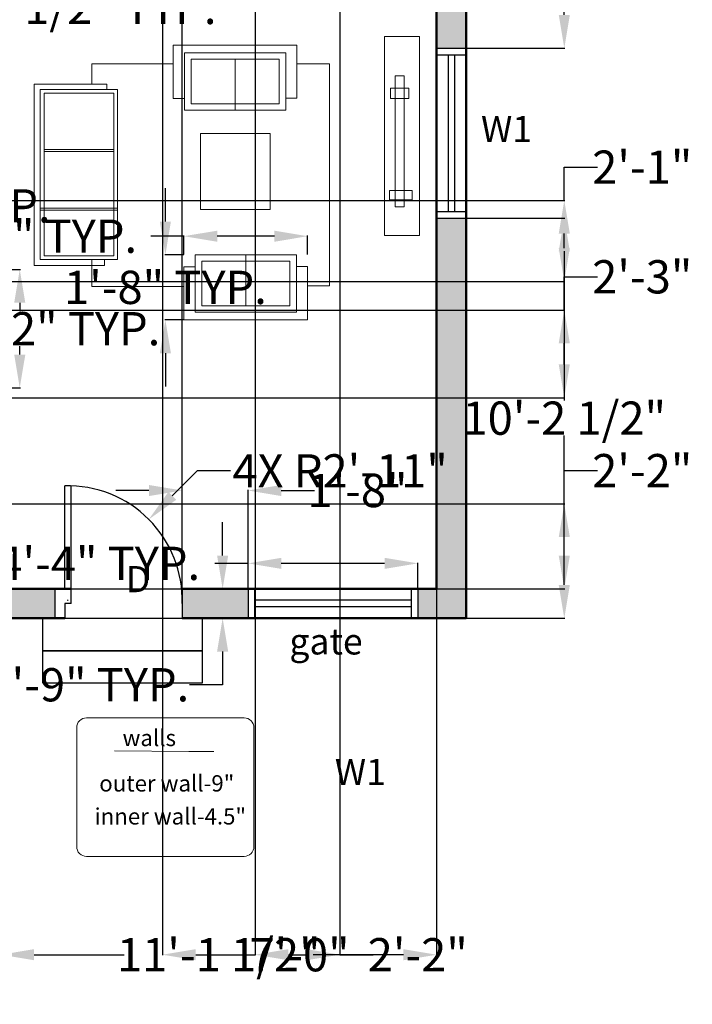
# Model space of a CAD drawing. Units: inches. Extents: x 2391 to 2964, y 130 to 798.
# Tile 2 of 4: x 2666 to 2872, y 130 to 431. Entities that reach past the tile are written whole.
import ezdxf

# ---------------------------------------------------------------- set-up
doc = ezdxf.new("R2010")
doc.units = ezdxf.units.IN
doc.header["$MEASUREMENT"] = 0
for name, color, linetype, lineweight in [('A-ANNO-DIMS', 2, 'Continuous', 18), ('A-ANNO-LEGN', 7, 'Continuous', 18), ('A-ANNO-TEXT', 7, 'Continuous', 18), ('A-DOOR', 3, 'Continuous', 25), ('A-FLOR-STRS', 7, 'Continuous', 30), ('A-FURN', 8, 'Continuous', 18), ('A-GLAZ', 4, 'Continuous', 25), ('A-WALL', 7, 'Continuous', 50)]:
    doc.layers.add(name, color=color, linetype=linetype, lineweight=lineweight)
doc.layers.add('A-WALL-PATT', color=11, linetype='Continuous', lineweight=13, true_color=0xf27172)
doc.styles.get("Standard").update_dxf_attribs({"font": 'arial.ttf'})
doc.dimstyles.get("Standard").update_dxf_attribs({"dimtxt": 10.18, "dimasz": 10.18, "dimexe": 0.18, "dimexo": 0.0625, "dimgap": 0.09, "dimtad": 0, "dimtih": 1, "dimtoh": 1, "dimdec": 0, "dimzin": 0, "dimdsep": 46, "dimlunit": 3, "dimtxsty": 'Standard', "dimcen": 0.09, "dimadec": 0, "dimazin": 0, "dimtfac": 1, "dimtdec": 0, "dimtofl": 0, "dimtmove": 0, "dimatfit": 3, "dimfxl": 1, "dimtolj": 1, "dimtzin": 0, "dimarcsym": 0})

# ---------------------------------------------------------------- blocks, each defined once
blk = doc.blocks.new('WIN-W1-48')
for p, q in [((0, 0), (0, 9)), ((2, 0), (2, 9)), ((50, 0), (50, 9)), ((52, 0), (52, 9)), ((2, 5.5), (50, 5.5)), ((2, 3.5), (50, 3.5))]:
    blk.add_line(p, q)
blk = doc.blocks.new('LOVESEAT')
for p, q in [((0, 3.57), (0, 19.95)), ((37.89, 19.95), (0, 19.95)), ((37.89, 19.95), (37.89, 3.71)), ((18.95, 15.6), (18.95, 0)), ((3.45, 3.57), (0, 3.57)), ((3.45, 3.57), (3.45, 3.57)), ((37.89, 3.71), (34.45, 3.71))]:
    blk.add_line(p, q)
for points in [[(3.45, 17.6), (34.45, 17.6), (34.45, 0), (3.45, 0)], [(5.45, 15.6), (32.45, 15.6), (32.45, 2), (5.45, 2)]]:
    blk.add_lwpolyline(points, close=True)
blk = doc.blocks.new('LEGEND-FRAME')
blk.add_line((11.62, 32.27), (34.31, 32.13))
blk.add_lwpolyline([(0, 39.41, -0.414214), (3, 42.41), (51.31, 42.41, -0.414214), (54.31, 39.41), (54.31, 3, -0.414214), (51.31, 0), (3, 0, -0.414214), (0, 3)], format="xyb", close=True)
blk = doc.blocks.new('*D15')
at = {"layer": 'A-ANNO-DIMS', "color": 0, "lineweight": -2, "transparency": 16777216}
for p, q in [((2735.63, 257.3), (2735.63, 265.22)), ((2787.63, 257.3), (2787.63, 265.22)), ((2735.63, 265.04), (2725.45, 265.04)), ((2777.45, 265.04), (2745.81, 265.04))]:
    blk.add_line(p, q, dxfattribs=at)
at = {"layer": 'A-ANNO-DIMS', "color": 0, "transparency": 16777216}
for points in [[(2745.81, 266.73), (2745.81, 263.34), (2735.63, 265.04)], [(2777.45, 266.73), (2777.45, 263.34), (2787.63, 265.04)]]:
    blk.add_solid(points, dxfattribs=at)
at = {"layer": 'Defpoints', "color": 0, "transparency": 16777216}
for p in [(2735.63, 265.04), (2735.63, 257.24), (2787.63, 257.24)]:
    blk.add_point(p, dxfattribs=at)
at = {"layer": 'A-ANNO-DIMS', "color": 0, "transparency": 16777216, "insert": (2654.62, 265.04), "char_height": 10.18, "attachment_point": 5}
blk.add_mtext('\\A1;W1 FRAME 4\'-4" TYP.', dxfattribs=at)
blk = doc.blocks.new('*D16')
at = {"layer": 'A-ANNO-DIMS', "color": 0, "lineweight": -2, "transparency": 16777216}
for p, q in [((2727.83, 267.42), (2727.83, 277.6)), ((2735.57, 257.24), (2727.65, 257.24)), ((2735.57, 248.24), (2727.65, 248.24)), ((2727.83, 238.06), (2727.83, 227.88)), ((2727.83, 227.88), (2717.65, 227.88))]:
    blk.add_line(p, q, dxfattribs=at)
at = {"layer": 'A-ANNO-DIMS', "color": 0, "transparency": 16777216}
for points in [[(2726.14, 267.42), (2729.53, 267.42), (2727.83, 257.24)], [(2726.14, 238.06), (2729.53, 238.06), (2727.83, 248.24)]]:
    blk.add_solid(points, dxfattribs=at)
at = {"layer": 'Defpoints', "color": 0, "transparency": 16777216}
for p in [(2735.63, 257.24), (2727.83, 248.24), (2735.63, 248.24)]:
    blk.add_point(p, dxfattribs=at)
at = {"layer": 'A-ANNO-DIMS', "color": 0, "transparency": 16777216, "insert": (2686.54, 227.88), "char_height": 10.18, "attachment_point": 5}
blk.add_mtext('\\A1;0\'-9" TYP.', dxfattribs=at)
blk = doc.blocks.new('*D18')
at = {"layer": 'A-ANNO-DIMS', "color": 0, "lineweight": -2, "transparency": 16777216}
for p, q in [((2659.96, 355.01), (2665.86, 355.01)), ((2665.68, 344.83), (2665.68, 342.23)), ((2665.68, 328.92), (2665.68, 331.52)), ((2659.96, 318.74), (2665.86, 318.74))]:
    blk.add_line(p, q, dxfattribs=at)
at = {"layer": 'A-ANNO-DIMS', "color": 0, "transparency": 16777216}
for points in [[(2663.98, 344.83), (2667.38, 344.83), (2665.68, 355.01)], [(2663.98, 328.92), (2667.38, 328.92), (2665.68, 318.74)]]:
    blk.add_solid(points, dxfattribs=at)
at = {"layer": 'Defpoints', "color": 0, "transparency": 16777216}
for p in [(2659.9, 355.01), (2665.68, 355.01), (2659.9, 318.74)]:
    blk.add_point(p, dxfattribs=at)
at = {"layer": 'A-ANNO-DIMS', "color": 0, "transparency": 16777216, "insert": (2665.68, 336.87), "char_height": 10.18, "attachment_point": 5}
blk.add_mtext('\\A1;3\'-0 1/2" TYP.', dxfattribs=at)
blk = doc.blocks.new('*D25')
at = {"layer": 'A-ANNO-DIMS', "color": 0, "lineweight": -2, "transparency": 16777216}
for p, q in [((2507.85, 435.2), (2497.67, 435.2)), ((2518.03, 436.55), (2518.03, 435.02)), ((2527.43, 436.55), (2527.43, 435.02)), ((2537.61, 435.2), (2547.79, 435.2))]:
    blk.add_line(p, q, dxfattribs=at)
at = {"layer": 'A-ANNO-DIMS', "color": 0, "transparency": 16777216}
for points in [[(2507.85, 436.9), (2507.85, 433.5), (2518.03, 435.2)], [(2537.61, 436.9), (2537.61, 433.5), (2527.43, 435.2)]]:
    blk.add_solid(points, dxfattribs=at)
at = {"layer": 'Defpoints', "color": 0, "transparency": 16777216}
for p in [(2518.03, 436.61), (2527.43, 436.61), (2527.43, 435.2)]:
    blk.add_point(p, dxfattribs=at)
at = {"layer": 'A-ANNO-DIMS', "color": 0, "transparency": 16777216, "insert": (2639.1, 435.2), "char_height": 10.18, "attachment_point": 5}
blk.add_mtext('\\A1;END TABLE C 0\'-9 1/2" TYP.', dxfattribs=at)
blk = doc.blocks.new('*D27')
at = {"layer": 'A-ANNO-DIMS', "color": 0, "lineweight": -2, "transparency": 16777216}
for p, q in [((2715.98, 365.18), (2705.8, 365.18)), ((2715.98, 359.56), (2715.98, 365.36)), ((2743.69, 365.18), (2726.16, 365.18)), ((2753.87, 359.56), (2753.87, 365.36))]:
    blk.add_line(p, q, dxfattribs=at)
at = {"layer": 'A-ANNO-DIMS', "color": 0, "transparency": 16777216}
for points in [[(2726.16, 366.87), (2726.16, 363.48), (2715.98, 365.18)], [(2743.69, 366.87), (2743.69, 363.48), (2753.87, 365.18)]]:
    blk.add_solid(points, dxfattribs=at)
at = {"layer": 'Defpoints', "color": 0, "transparency": 16777216}
for p in [(2715.98, 365.18), (2715.98, 359.49), (2753.87, 359.49)]:
    blk.add_point(p, dxfattribs=at)
at = {"layer": 'A-ANNO-DIMS', "color": 0, "transparency": 16777216, "insert": (2635.39, 365.18), "char_height": 10.18, "attachment_point": 5}
blk.add_mtext('\\A1;LOVESEAT 3\'-2" TYP.', dxfattribs=at)
blk = doc.blocks.new('*D28')
at = {"layer": 'A-ANNO-DIMS', "color": 0, "lineweight": -2, "transparency": 16777216}
for p, q in [((2710.3, 369.67), (2710.3, 379.85)), ((2715.92, 359.49), (2710.12, 359.49)), ((2715.92, 339.54), (2710.12, 339.54)), ((2710.3, 329.36), (2710.3, 319.18))]:
    blk.add_line(p, q, dxfattribs=at)
at = {"layer": 'A-ANNO-DIMS', "color": 0, "transparency": 16777216}
for points in [[(2708.6, 369.67), (2711.99, 369.67), (2710.3, 359.49)], [(2708.6, 329.36), (2711.99, 329.36), (2710.3, 339.54)]]:
    blk.add_solid(points, dxfattribs=at)
at = {"layer": 'Defpoints', "color": 0, "transparency": 16777216}
for p in [(2715.98, 359.49), (2710.3, 339.54), (2715.98, 339.54)]:
    blk.add_point(p, dxfattribs=at)
at = {"layer": 'A-ANNO-DIMS', "color": 0, "transparency": 16777216, "insert": (2710.3, 349.52), "char_height": 10.18, "attachment_point": 5}
blk.add_mtext('\\A1;1\'-8" TYP.', dxfattribs=at)
blk = doc.blocks.new('*D29')
at = {"layer": 'A-ANNO-DIMS', "color": 0, "lineweight": -2, "transparency": 16777216}
for p, q in [((2515.72, 374.47), (2505.54, 374.47)), ((2525.9, 373.66), (2525.9, 374.65)), ((2531.76, 373.66), (2531.76, 374.65)), ((2541.94, 374.47), (2552.12, 374.47))]:
    blk.add_line(p, q, dxfattribs=at)
at = {"layer": 'A-ANNO-DIMS', "color": 0, "transparency": 16777216}
for points in [[(2515.72, 376.17), (2515.72, 372.78), (2525.9, 374.47)], [(2541.94, 376.17), (2541.94, 372.78), (2531.76, 374.47)]]:
    blk.add_solid(points, dxfattribs=at)
at = {"layer": 'Defpoints', "color": 0, "transparency": 16777216}
for p in [(2531.76, 374.47), (2525.9, 373.59), (2531.76, 373.59)]:
    blk.add_point(p, dxfattribs=at)
at = {"layer": 'A-ANNO-DIMS', "color": 0, "transparency": 16777216, "insert": (2615.01, 374.47), "char_height": 10.18, "attachment_point": 5}
blk.add_mtext('\\A1;BURNER 0\'-6" TYP.', dxfattribs=at)
blk = doc.blocks.new('*D33')
at = {"layer": 'A-ANNO-DIMS', "color": 0, "lineweight": -2, "transparency": 16777216}
for p, q in [((2659.9, 743.17), (2659.9, 145.07)), ((2793.4, 743.17), (2793.4, 145.07)), ((2670.08, 145.25), (2697.69, 145.25)), ((2783.22, 145.25), (2755.61, 145.25))]:
    blk.add_line(p, q, dxfattribs=at)
at = {"layer": 'A-ANNO-DIMS', "color": 0, "transparency": 16777216}
for points in [[(2670.08, 146.95), (2670.08, 143.56), (2659.9, 145.25)], [(2783.22, 146.95), (2783.22, 143.56), (2793.4, 145.25)]]:
    blk.add_solid(points, dxfattribs=at)
at = {"layer": 'Defpoints', "color": 0, "transparency": 16777216}
for p in [(2659.9, 743.24), (2793.4, 743.24), (2793.4, 145.25)]:
    blk.add_point(p, dxfattribs=at)
at = {"layer": 'A-ANNO-DIMS', "color": 0, "transparency": 16777216, "insert": (2726.65, 145.25), "char_height": 10.18, "attachment_point": 5}
blk.add_mtext('\\A1;11\'-1 1/2"', dxfattribs=at)
blk = doc.blocks.new('*D36')
at = {"layer": 'A-ANNO-DIMS', "color": 0, "lineweight": -2, "transparency": 16777216}
for p, q in [((2709.4, 594.67), (2709.4, 145.07)), ((2793.4, 594.67), (2793.4, 145.07)), ((2719.58, 145.25), (2737.82, 145.25)), ((2783.22, 145.25), (2764.98, 145.25))]:
    blk.add_line(p, q, dxfattribs=at)
at = {"layer": 'A-ANNO-DIMS', "color": 0, "transparency": 16777216}
for points in [[(2719.58, 146.95), (2719.58, 143.56), (2709.4, 145.25)], [(2783.22, 146.95), (2783.22, 143.56), (2793.4, 145.25)]]:
    blk.add_solid(points, dxfattribs=at)
at = {"layer": 'Defpoints', "color": 0, "transparency": 16777216}
for p in [(2709.4, 594.74), (2793.4, 594.74), (2793.4, 145.25)]:
    blk.add_point(p, dxfattribs=at)
at = {"layer": 'A-ANNO-DIMS', "color": 0, "transparency": 16777216, "insert": (2751.4, 145.25), "char_height": 10.18, "attachment_point": 5}
blk.add_mtext('\\A1;7\'-0"', dxfattribs=at)
blk = doc.blocks.new('*D42')
at = {"layer": 'A-ANNO-DIMS', "color": 0, "lineweight": -2, "transparency": 16777216}
for p, q in [((2802.46, 370.74), (2832.68, 370.74)), ((2832.5, 360.56), (2832.5, 314.84)), ((2832.5, 258.42), (2832.5, 304.13)), ((2802.46, 248.24), (2832.68, 248.24))]:
    blk.add_line(p, q, dxfattribs=at)
at = {"layer": 'A-ANNO-DIMS', "color": 0, "transparency": 16777216}
for points in [[(2830.8, 360.56), (2834.2, 360.56), (2832.5, 370.74)], [(2830.8, 258.42), (2834.2, 258.42), (2832.5, 248.24)]]:
    blk.add_solid(points, dxfattribs=at)
at = {"layer": 'Defpoints', "color": 0, "transparency": 16777216}
for p in [(2802.4, 370.74), (2832.5, 370.74), (2802.4, 248.24)]:
    blk.add_point(p, dxfattribs=at)
at = {"layer": 'A-ANNO-DIMS', "color": 0, "transparency": 16777216, "insert": (2832.5, 309.49), "char_height": 10.18, "attachment_point": 5}
blk.add_mtext('\\A1;10\'-2 1/2"', dxfattribs=at)
blk = doc.blocks.new('*D43')
at = {"layer": 'A-ANNO-DIMS', "color": 0, "lineweight": -2, "transparency": 16777216}
for p, q in [((2802.46, 555.74), (2832.68, 555.74)), ((2832.5, 545.56), (2832.5, 494.44)), ((2832.5, 432.92), (2832.5, 484.03)), ((2802.46, 422.74), (2832.68, 422.74))]:
    blk.add_line(p, q, dxfattribs=at)
at = {"layer": 'A-ANNO-DIMS', "color": 0, "transparency": 16777216}
for points in [[(2830.8, 545.56), (2834.2, 545.56), (2832.5, 555.74)], [(2830.8, 432.92), (2834.2, 432.92), (2832.5, 422.74)]]:
    blk.add_solid(points, dxfattribs=at)
at = {"layer": 'Defpoints', "color": 0, "transparency": 16777216}
for p in [(2802.4, 555.74), (2832.5, 555.74), (2802.4, 422.74)]:
    blk.add_point(p, dxfattribs=at)
at = {"layer": 'A-ANNO-DIMS', "color": 0, "transparency": 16777216, "insert": (2832.5, 489.24), "char_height": 10.18, "attachment_point": 5}
blk.add_mtext('\\A1;11\'-1"', dxfattribs=at)
blk = doc.blocks.new('*D44')
at = {"layer": 'A-ANNO-DIMS', "color": 0, "lineweight": -2, "transparency": 16777216}
for p, q in [((2715.45, 257.3), (2715.45, 782.52)), ((2725.63, 782.34), (2740.78, 782.34)), ((2783.22, 782.34), (2768.07, 782.34)), ((2793.4, 257.3), (2793.4, 782.52))]:
    blk.add_line(p, q, dxfattribs=at)
at = {"layer": 'A-ANNO-DIMS', "color": 0, "transparency": 16777216}
for points in [[(2725.63, 784.03), (2725.63, 780.64), (2715.45, 782.34)], [(2783.22, 784.03), (2783.22, 780.64), (2793.4, 782.34)]]:
    blk.add_solid(points, dxfattribs=at)
at = {"layer": 'Defpoints', "color": 0, "transparency": 16777216}
for p in [(2793.4, 782.34), (2715.45, 257.24), (2793.4, 257.24)]:
    blk.add_point(p, dxfattribs=at)
at = {"layer": 'A-ANNO-DIMS', "color": 0, "transparency": 16777216, "insert": (2754.42, 782.34), "char_height": 10.18, "attachment_point": 5}
blk.add_mtext('\\A1;6\'-6"', dxfattribs=at)
blk = doc.blocks.new('*D45')
at = {"layer": 'A-ANNO-DIMS', "color": 0, "lineweight": -2, "transparency": 16777216}
for p, q in [((2705.27, 287.34), (2695.09, 287.34)), ((2715.45, 257.3), (2715.45, 287.52)), ((2735.63, 257.3), (2735.63, 287.52)), ((2745.81, 287.34), (2755.99, 287.34))]:
    blk.add_line(p, q, dxfattribs=at)
at = {"layer": 'A-ANNO-DIMS', "color": 0, "transparency": 16777216}
for points in [[(2705.27, 289.03), (2705.27, 285.64), (2715.45, 287.34)], [(2745.81, 289.03), (2745.81, 285.64), (2735.63, 287.34)]]:
    blk.add_solid(points, dxfattribs=at)
at = {"layer": 'Defpoints', "color": 0, "transparency": 16777216}
for p in [(2735.63, 287.34), (2715.45, 257.24), (2735.63, 257.24)]:
    blk.add_point(p, dxfattribs=at)
at = {"layer": 'A-ANNO-DIMS', "color": 0, "transparency": 16777216, "insert": (2769.13, 287.34), "char_height": 10.18, "attachment_point": 5}
blk.add_mtext('\\A1;1\'-8"', dxfattribs=at)
blk = doc.blocks.new('*D46')
at = {"layer": 'A-ANNO-DIMS', "color": 0, "lineweight": -2, "transparency": 16777216}
for p, q in [((2737.79, 536.17), (2737.79, 145.07)), ((2763.73, 536.17), (2763.73, 145.07)), ((2747.97, 145.25), (2753.55, 145.25)), ((2763.73, 145.25), (2773.91, 145.25))]:
    blk.add_line(p, q, dxfattribs=at)
at = {"layer": 'A-ANNO-DIMS', "color": 0, "transparency": 16777216}
for points in [[(2747.97, 146.95), (2747.97, 143.56), (2737.79, 145.25)], [(2753.55, 146.95), (2753.55, 143.56), (2763.73, 145.25)]]:
    blk.add_solid(points, dxfattribs=at)
at = {"layer": 'Defpoints', "color": 0, "transparency": 16777216}
for p in [(2737.79, 536.24), (2763.73, 536.24), (2763.73, 145.25)]:
    blk.add_point(p, dxfattribs=at)
at = {"layer": 'A-ANNO-DIMS', "color": 0, "transparency": 16777216, "insert": (2787.61, 145.25), "char_height": 10.18, "attachment_point": 5}
blk.add_mtext('\\A1;2\'-2"', dxfattribs=at)
blk = doc.blocks.new('*D51')
at = {"layer": 'A-ANNO-DIMS', "color": 0, "lineweight": -2, "transparency": 16777216}
for p, q in [((2832.5, 342.57), (2832.5, 352.75)), ((2832.5, 352.75), (2842.68, 352.75)), ((2594.69, 342.57), (2832.68, 342.57)), ((2832.5, 325.92), (2832.5, 332.39)), ((2594.69, 315.74), (2832.68, 315.74))]:
    blk.add_line(p, q, dxfattribs=at)
at = {"layer": 'A-ANNO-DIMS', "color": 0, "transparency": 16777216}
for points in [[(2830.8, 332.39), (2834.2, 332.39), (2832.5, 342.57)], [(2830.8, 325.92), (2834.2, 325.92), (2832.5, 315.74)]]:
    blk.add_solid(points, dxfattribs=at)
at = {"layer": 'Defpoints', "color": 0, "transparency": 16777216}
for p in [(2594.63, 342.57), (2832.5, 342.57), (2594.63, 315.74)]:
    blk.add_point(p, dxfattribs=at)
at = {"layer": 'A-ANNO-DIMS', "color": 0, "transparency": 16777216, "insert": (2856.39, 352.75), "char_height": 10.18, "attachment_point": 5}
blk.add_mtext('\\A1;2\'-3"', dxfattribs=at)
blk = doc.blocks.new('*D52')
at = {"layer": 'A-ANNO-DIMS', "color": 0, "lineweight": -2, "transparency": 16777216}
for p, q in [((2615.22, 782.34), (2605.04, 782.34)), ((2625.4, 311.3), (2625.4, 782.52)), ((2635.4, 311.3), (2635.4, 782.52)), ((2645.58, 782.34), (2655.76, 782.34))]:
    blk.add_line(p, q, dxfattribs=at)
at = {"layer": 'A-ANNO-DIMS', "color": 0, "transparency": 16777216}
for points in [[(2615.22, 784.03), (2615.22, 780.64), (2625.4, 782.34)], [(2645.58, 784.03), (2645.58, 780.64), (2635.4, 782.34)]]:
    blk.add_solid(points, dxfattribs=at)
at = {"layer": 'Defpoints', "color": 0, "transparency": 16777216}
for p in [(2635.4, 782.34), (2625.4, 311.24), (2635.4, 311.24)]:
    blk.add_point(p, dxfattribs=at)
at = {"layer": 'A-ANNO-DIMS', "color": 0, "transparency": 16777216, "insert": (2673.33, 782.34), "char_height": 10.18, "attachment_point": 5}
blk.add_mtext('\\A1;0\'-10"', dxfattribs=at)
blk = doc.blocks.new('*D53')
at = {"layer": 'A-ANNO-DIMS', "color": 0, "lineweight": -2, "transparency": 16777216}
for p, q in [((2832.5, 283.24), (2832.5, 293.42)), ((2832.5, 293.42), (2842.68, 293.42)), ((2645.46, 283.24), (2832.68, 283.24)), ((2832.5, 267.42), (2832.5, 273.06)), ((2645.46, 257.24), (2832.68, 257.24))]:
    blk.add_line(p, q, dxfattribs=at)
at = {"layer": 'A-ANNO-DIMS', "color": 0, "transparency": 16777216}
for points in [[(2830.8, 273.06), (2834.2, 273.06), (2832.5, 283.24)], [(2830.8, 267.42), (2834.2, 267.42), (2832.5, 257.24)]]:
    blk.add_solid(points, dxfattribs=at)
at = {"layer": 'Defpoints', "color": 0, "transparency": 16777216}
for p in [(2645.4, 283.24), (2832.5, 283.24), (2645.4, 257.24)]:
    blk.add_point(p, dxfattribs=at)
at = {"layer": 'A-ANNO-DIMS', "color": 0, "transparency": 16777216, "insert": (2856.39, 293.42), "char_height": 10.18, "attachment_point": 5}
blk.add_mtext('\\A1;2\'-2"', dxfattribs=at)
blk = doc.blocks.new('*D57')
at = {"layer": 'A-ANNO-DIMS', "color": 0, "lineweight": -2, "transparency": 16777216}
for p, q in [((2832.5, 376.14), (2832.5, 386.32)), ((2832.5, 386.32), (2842.68, 386.32)), ((2534.83, 376.14), (2832.68, 376.14)), ((2832.5, 361.53), (2832.5, 365.96)), ((2534.83, 351.35), (2832.68, 351.35))]:
    blk.add_line(p, q, dxfattribs=at)
at = {"layer": 'A-ANNO-DIMS', "color": 0, "transparency": 16777216}
for points in [[(2830.8, 365.96), (2834.2, 365.96), (2832.5, 376.14)], [(2830.8, 361.53), (2834.2, 361.53), (2832.5, 351.35)]]:
    blk.add_solid(points, dxfattribs=at)
at = {"layer": 'Defpoints', "color": 0, "transparency": 16777216}
for p in [(2534.77, 376.14), (2832.5, 376.14), (2534.77, 351.35)]:
    blk.add_point(p, dxfattribs=at)
at = {"layer": 'A-ANNO-DIMS', "color": 0, "transparency": 16777216, "insert": (2856.39, 386.32), "char_height": 10.18, "attachment_point": 5}
blk.add_mtext('\\A1;2\'-1"', dxfattribs=at)
blk = doc.blocks.new('*D60')
at = {"layer": 'A-ANNO-DIMS', "color": 0, "lineweight": -2, "transparency": 16777216}
for p, q in [((2720.06, 293.35), (2712.4, 285.69)), ((2730.24, 293.35), (2720.06, 293.35)), ((2680.36, 253.74), (2680.54, 253.74)), ((2680.45, 253.65), (2680.45, 253.83))]:
    blk.add_line(p, q, dxfattribs=at)
at = {"layer": 'A-ANNO-DIMS', "color": 0, "transparency": 16777216}
blk.add_solid([(2711.2, 286.89), (2713.6, 284.49), (2705.21, 278.49)], dxfattribs=at)
at = {"layer": 'Defpoints', "color": 0, "transparency": 16777216}
for p in [(2705.21, 278.49), (2680.45, 253.74)]:
    blk.add_point(p, dxfattribs=at)
at = {"layer": 'A-ANNO-DIMS', "color": 0, "transparency": 16777216, "insert": (2763.83, 293.35), "char_height": 10.18, "attachment_point": 5}
blk.add_mtext('\\A1;4X R2\'-11"', dxfattribs=at)

msp = doc.modelspace()

# ---------------------------------------------------------------- hatches: boundary and pattern name
at = {"layer": 'A-WALL-PATT'}
h = msp.add_hatch(color=256, dxfattribs=at)
h.dxf.hatch_style = 1
h.paths.add_polyline_path([(2557.4, 752.24), (2502.4, 752.24), (2502.4, 579.74), (2511.4, 579.74), (2511.4, 594.74), (2595.4, 594.74), (2599.9, 594.74), (2616.4, 594.74), (2616.4, 596.99, -0.014283), (2616.4, 598.99), (2616.4, 599.24), (2511.4, 599.24), (2511.4, 743.24), (2557.4, 743.24)])
h.paths.add_polyline_path([(2700.65, 752.24), (2609.4, 752.24), (2609.4, 743.24), (2655.4, 743.24), (2655.4, 599.24), (2650.4, 599.24), (2650.4, 596.99), (2652.4, 596.99), (2652.4, 594.74), (2662.9, 594.74), (2662.9, 596.99), (2664.9, 596.99), (2664.9, 599.24), (2659.9, 599.24), (2659.9, 743.24), (2700.65, 743.24)])
h.paths.add_polyline_path([(2802.4, 752.24), (2752.65, 752.24), (2752.65, 743.24), (2793.4, 743.24), (2793.4, 599.24), (2698.9, 599.24), (2698.9, 598.99, -0.014283), (2698.9, 596.99), (2698.9, 594.74), (2704.9, 594.74), (2704.9, 536.24), (2737.79, 536.24), (2737.79, 540.74), (2709.4, 540.74), (2709.4, 594.74), (2793.4, 594.74), (2793.4, 581.74), (2802.4, 581.74)])
h.paths.add_polyline_path([(2511.4, 444.24), (2502.4, 444.24), (2502.4, 383.74), (2511.4, 383.74), (2511.4, 399.74), (2655.4, 399.74), (2655.4, 354.74), (2655.65, 354.74, -0.014283), (2657.65, 354.74), (2659.9, 354.74), (2659.9, 407.24), (2657.65, 407.24), (2657.65, 409.24), (2655.4, 409.24), (2655.4, 404.24), (2511.4, 404.24)])
h.paths.add_polyline_path([(2511.4, 536.24), (2599.9, 536.24), (2655.4, 536.24), (2655.4, 443.24), (2655.65, 443.24, -0.014283), (2657.65, 443.24), (2659.9, 443.24), (2659.9, 540.74), (2599.9, 540.74), (2599.9, 555.74), (2597.65, 555.74, -0.014283), (2595.65, 555.74), (2595.4, 555.74), (2595.4, 540.74), (2511.4, 540.74), (2511.4, 555.74), (2502.4, 555.74), (2502.4, 496.24), (2511.4, 496.24), (2511.4, 503.82)])
h.paths.add_polyline_path([(2676.45, 257.24), (2511.4, 257.24), (2511.4, 311.24), (2659.9, 311.24), (2659.9, 318.74), (2657.65, 318.74), (2657.65, 320.74), (2655.4, 320.74), (2655.4, 315.74), (2511.4, 315.74), (2511.4, 331.74), (2502.4, 331.74), (2502.4, 248.24), (2676.45, 248.24)])
h.paths.add_polyline_path([(2802.4, 370.74), (2793.4, 370.74), (2793.4, 257.24), (2787.63, 257.24), (2787.63, 248.24), (2802.4, 248.24)])
h.paths.add_polyline_path([(2735.63, 257.24), (2715.45, 257.24), (2715.45, 254.74, -0.014283), (2715.45, 252.74), (2715.45, 248.24), (2721.55, 248.24), (2735.63, 248.24)])
h.paths.add_polyline_path([(2802.4, 553.74), (2793.4, 553.74), (2793.4, 540.74), (2763.73, 540.74), (2763.73, 536.24), (2793.4, 536.24), (2793.4, 422.74), (2802.4, 422.74)])

# ---------------------------------------------------------------- linework, layer by layer
at = {"layer": 'A-ANNO-LEGN'}
msp.add_line((2717.43, 207.48), (2725.17, 207.43), dxfattribs=at)
at = {"layer": 'A-DOOR'}
for p, q in [((2679.45, 257.24), (2679.45, 288.74)), ((2681.45, 252.74), (2681.45, 288.74)), ((2676.45, 257.24), (2676.45, 248.24)), ((2715.45, 257.24), (2715.45, 248.24)), ((2679.45, 252.74), (2679.45, 248.24)), ((2681.45, 252.74), (2679.45, 252.74))]:
    msp.add_line(p, q, dxfattribs=at)
msp.add_arc((2680.45, 253.74), 35.01, 358.3634, 91.6366, dxfattribs=at)
at = {"layer": 'A-FLOR-STRS'}
for points in [[(2672.7, 248.24), (2721.55, 248.24), (2721.55, 238.28), (2672.7, 238.28)], [(2672.7, 238.28), (2721.55, 238.28), (2721.55, 228.32), (2672.7, 228.32)]]:
    msp.add_lwpolyline(points, close=True, dxfattribs=at)
at = {"layer": 'A-FURN'}
for p, q in [((2687.77, 411.7), (2687.77, 417.91)), ((2687.77, 417.91), (2712.72, 417.91)), ((2750.61, 417.91), (2755.38, 417.91)), ((2760.53, 417.91), (2755.38, 417.91)), ((2760.53, 356.75), (2760.53, 417.91)), ((2670.14, 356.21), (2670.14, 411.7)), ((2670.14, 411.7), (2692.37, 411.7)), ((2692.37, 411.7), (2692.37, 410.11)), ((2694.5, 391.7), (2673.11, 391.7)), ((2694.5, 391.14), (2673.11, 391.14)), ((2695.64, 373.72), (2671.98, 373.72)), ((2695.64, 373.15), (2671.98, 373.15)), ((2691.64, 356.21), (2670.14, 356.21)), ((2687.77, 358.02), (2687.77, 349.83)), ((2691.64, 358.02), (2691.64, 356.21)), ((2760.53, 349.95), (2760.53, 356.75)), ((2687.77, 349.83), (2715.98, 349.83)), ((2753.87, 349.95), (2760.53, 349.95))]:
    msp.add_line(p, q, dxfattribs=at)
for points in [[(2788.12, 426.29), (2777.46, 426.29), (2777.46, 365.42), (2788.12, 365.42)], [(2780.7, 414.25), (2783.48, 414.25), (2783.48, 374.21), (2780.7, 374.21)], [(2695.64, 358.02), (2671.98, 358.02), (2671.98, 410.11), (2695.64, 410.11)], [(2779.26, 410.48), (2784.88, 410.48), (2784.88, 407.35), (2779.26, 407.35)], [(2694.5, 359.15), (2673.11, 359.15), (2673.11, 408.98), (2694.5, 408.98)], [(2721.09, 396.66), (2742.36, 396.66), (2742.36, 373.38), (2721.09, 373.38)], [(2778.92, 379.19), (2785.87, 379.19), (2785.87, 376.32), (2778.92, 376.32)]]:
    msp.add_lwpolyline(points, close=True, dxfattribs=at)
at = {"layer": 'A-WALL'}
for p, q in [((2802.4, 752.24), (2802.4, 248.24)), ((2793.4, 536.24), (2793.4, 257.24)), ((2681.45, 257.24), (2511.4, 257.24)), ((2793.4, 257.24), (2715.29, 257.24)), ((2679.45, 248.24), (2502.4, 248.24)), ((2802.4, 248.24), (2715.45, 248.24))]:
    msp.add_line(p, q, dxfattribs=at)

# ---------------------------------------------------------------- block references
at = {"layer": 'A-ANNO-LEGN'}
msp.add_blockref('LEGEND-FRAME', (2683.12, 175.35), dxfattribs=at)
at = {"layer": 'A-FURN'}
msp.add_blockref('LOVESEAT', (2712.72, 403.72), dxfattribs=at)
at = {"layer": 'A-FURN', "rotation": 180}
msp.add_blockref('LOVESEAT', (2753.87, 359.49), dxfattribs=at)
at = {"layer": 'A-GLAZ'}
for p, rotation in [((2793.4, 422.73), 269.999999999998), ((2787.63, 257.24), 180)]:
    msp.add_blockref('WIN-W1-48', p, dxfattribs=dict(at, rotation=rotation))

# ---------------------------------------------------------------- texts
at = {"layer": 'A-ANNO-TEXT', "attachment_point": 1}
for s, width, insert, char_height in [('W1', 35.9617, (2806.99, 401.98), 8), ('D', 35.9617, (2698.19, 264.21), 8), ('gate', 35.9617, (2748.27, 245.15), 8), ('walls', 20.8895, (2697.17, 214.11), 5), ('W1', 35.9617, (2762.2, 205.2), 8), ('outer wall-9"', 48.0836, (2690.03, 200.2), 5), ('inner wall-4.5"', 61.4078, (2688.59, 190.1), 5)]:
    msp.add_mtext_dynamic_manual_height_columns(s, width=width, gutter_width=1, heights=[0], dxfattribs=dict(at, insert=insert, char_height=char_height))

# ---------------------------------------------------------------- dimensions: what is measured, and where the dimension line sits
at = {"layer": 'A-ANNO-DIMS'}
for base, p1, p2, picture, middle in [((2635.4, 782.34), (2625.4, 311.24), (2635.4, 311.24), '*D52', (2673.33, 782.34)), ((2793.3997, 782.3351), (2715.4471, 257.2351), (2793.3997, 257.2351), '*D44', (2754.4234, 782.3351)), ((2793.4, 145.25), (2659.9, 743.24), (2793.4, 743.24), '*D33', (2726.65, 145.25)), ((2793.4, 145.25), (2709.4, 594.74), (2793.4, 594.74), '*D36', (2751.4, 145.25)), ((2763.73, 145.25), (2737.79, 536.24), (2763.73, 536.24), '*D46', (2787.61, 145.25)), ((2735.63, 287.34), (2715.45, 257.24), (2735.63, 257.24), '*D45', (2769.13, 287.34))]:
    dim = msp.add_linear_dim(base=base, p1=p1, p2=p2, dimstyle='Standard', override={"dimdec": 1, "dimlfac": 1, "dimrnd": 0, "dimzin": 1, "dimdsep": 46, "dimlunit": 4, "dimfrac": 2}, dxfattribs=at)
    dim.commit()
    dim.dimension.update_dxf_attribs({"geometry": picture, "text_midpoint": middle})
for base, p1, p2, picture, middle in [((2832.5, 555.74), (2802.4, 422.74), (2802.4, 555.74), '*D43', (2832.5, 489.24)), ((2832.5, 376.14), (2534.77, 351.35), (2534.77, 376.14), '*D57', (2856.39, 386.32)), ((2832.5, 370.74), (2802.4, 248.24), (2802.4, 370.74), '*D42', (2832.5, 309.49)), ((2832.5, 342.57), (2594.63, 315.74), (2594.63, 342.57), '*D51', (2856.39, 352.75)), ((2832.5, 283.24), (2645.4, 257.24), (2645.4, 283.24), '*D53', (2856.39, 293.42))]:
    dim = msp.add_linear_dim(base=base, p1=p1, p2=p2, angle=90, dimstyle='Standard', override={"dimdec": 1, "dimlfac": 1, "dimrnd": 0, "dimzin": 1, "dimdsep": 46, "dimlunit": 4, "dimfrac": 2}, dxfattribs=at)
    dim.commit()
    dim.dimension.update_dxf_attribs({"geometry": picture, "text_midpoint": middle})
for base, p1, p2, text, picture, middle in [((2527.43, 435.2), (2518.03, 436.61), (2527.43, 436.61), 'END TABLE C <> TYP.', '*D25', (2639.1, 435.2)), ((2531.76, 374.47), (2525.9, 373.59), (2531.76, 373.59), 'BURNER <> TYP.', '*D29', (2615.01, 374.47))]:
    dim = msp.add_linear_dim(base=base, p1=p1, p2=p2, text=text, dimstyle='Standard', override={"dimdec": 1, "dimlfac": 1, "dimrnd": 0, "dimzin": 1, "dimdsep": 46, "dimlunit": 4, "dimfrac": 2}, dxfattribs=at)
    dim.commit()
    dim.dimension.update_dxf_attribs({"geometry": picture, "text_midpoint": middle})
for base, p1, p2, angle, text, picture, middle in [((2715.98, 365.18), (2753.87, 359.49), (2715.98, 359.49), 180, 'LOVESEAT <> TYP.', '*D27', (2635.39, 365.18)), ((2710.2967, 339.542), (2715.9797, 359.4941), (2715.9797, 339.542), 270, '<> TYP.', '*D28', (2710.2967, 349.5181)), ((2665.68, 355.01), (2659.9, 318.74), (2659.9, 355.01), 90, '<> TYP.', '*D18', (2665.68, 336.87)), ((2735.63, 265.04), (2787.63, 257.24), (2735.63, 257.24), 180, 'W1 FRAME <> TYP.', '*D15', (2654.62, 265.04)), ((2727.83, 248.24), (2735.63, 257.24), (2735.63, 248.24), 270, '<> TYP.', '*D16', (2686.54, 227.88))]:
    dim = msp.add_linear_dim(base=base, p1=p1, p2=p2, angle=angle, text=text, dimstyle='Standard', override={"dimdec": 1, "dimlfac": 1, "dimrnd": 0, "dimzin": 1, "dimdsep": 46, "dimlunit": 4, "dimfrac": 2}, dxfattribs=at)
    dim.commit()
    dim.dimension.update_dxf_attribs({"geometry": picture, "text_midpoint": middle})
dim = msp.add_radius_dim(center=(2680.45, 253.74), mpoint=(2705.21, 278.49), text='4X <>', dimstyle='Standard', override={"dimdec": 1, "dimlfac": 1, "dimrnd": 0, "dimzin": 1, "dimdsep": 46, "dimlunit": 4, "dimfrac": 2}, dxfattribs=at)
dim.commit()
dim.dimension.update_dxf_attribs({"geometry": '*D60', "text_midpoint": (2763.83, 293.35), "dimtype": 164})

doc.saveas('drawing.dxf')
